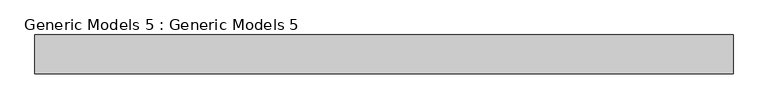
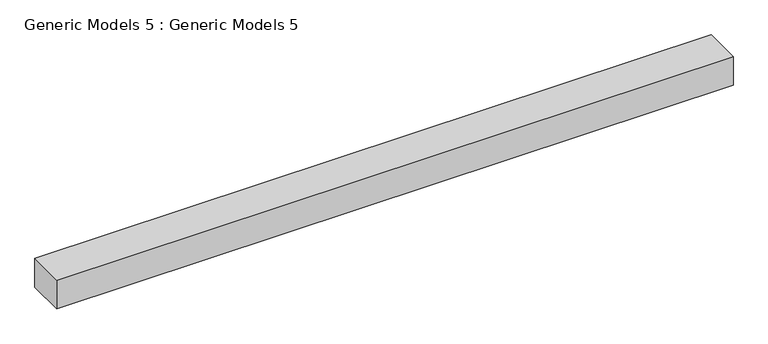
"""IFC4 building model written with IfcOpenShell, lengths in millimetres: proxy geometry, Generic Models 5 : Generic Models 5."""

from ifc_helpers import new_model, si_unit, frame, origin, place, context, project, spatial, polyline, outline, extrude, source, transform, mapped, element, save


def generic_models_5_generic_models_5_6f0b94fe(model_context):
    return source(origin(), model_context, "Body", "SweptSolid", [
        extrude(outline(polyline([(-8209.088074, -21454.4420973), (-8209.088074, -20845.7985361), (2694.3646622, -20845.7985361), (2694.3646622, -21454.4420973), (-8209.088074, -21454.4420973)])), frame((0.0, 0.0, 22699.4246611), z_axis=(0.0, 0.0, 1.0), x_axis=(1.0, 0.0, 0.0)), (0.0, 0.0, 1.0), 487.7923248),
    ])


if __name__ == "__main__":
    model = new_model("IFC4")
    model_context = context("Model", 3, world=origin())
    ifc_project = project(units=[si_unit("LENGTHUNIT", "METRE", prefix="MILLI")], contexts=[model_context])
    site = spatial("IfcSite", under=ifc_project)
    building = spatial("IfcBuilding", under=site)
    placement = place(None, origin())
    generic_models_5_generic_models_5_shape = generic_models_5_generic_models_5_6f0b94fe(model_context)
    element("IfcBuildingElementProxy", 1, Name="Generic Models 5 : Generic Models 5", ObjectType="Generic Models 5 : Generic Models 5", at=placement, inside=building, context=model_context, shape_type="MappedRepresentation", body=[
        mapped(generic_models_5_generic_models_5_shape, transform((0.0, 0.0, 0.0), x_axis=(1.0, 0.0, 0.0), y_axis=(0.0, 1.0, 0.0), z_axis=(0.0, 0.0, 1.0))),
    ])
    save(model, "model.ifc")
